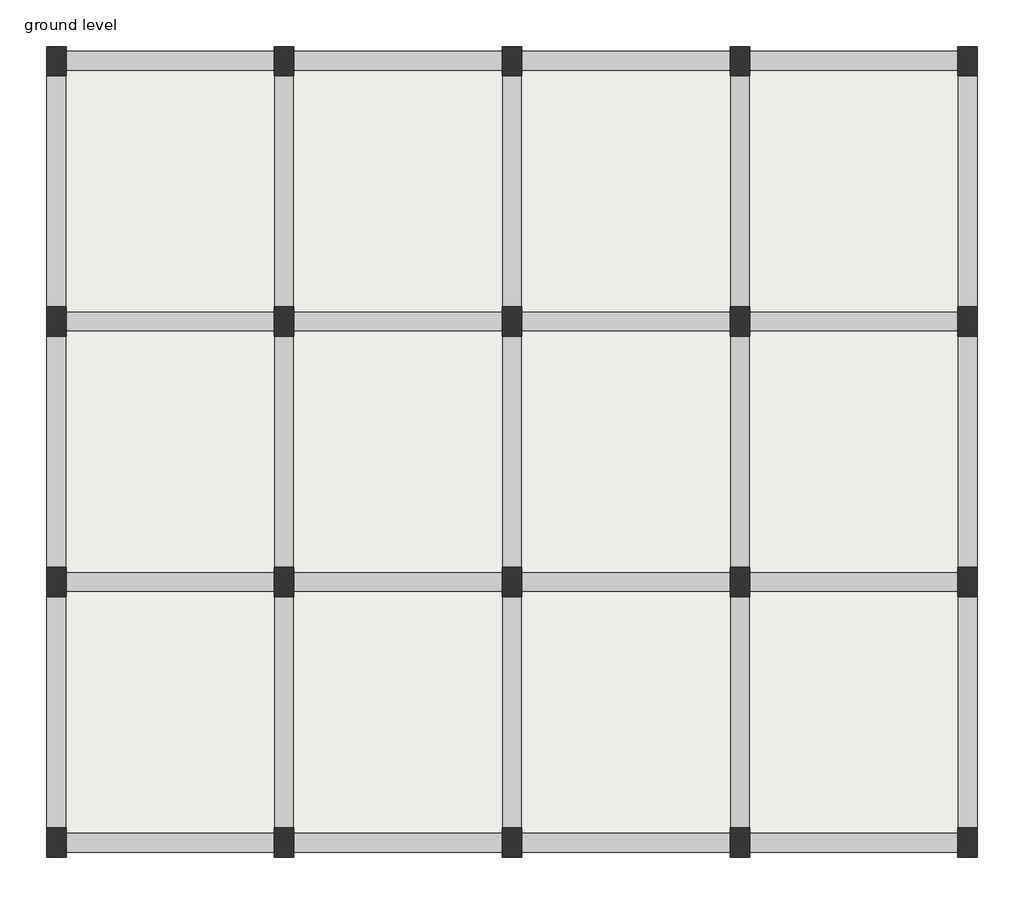
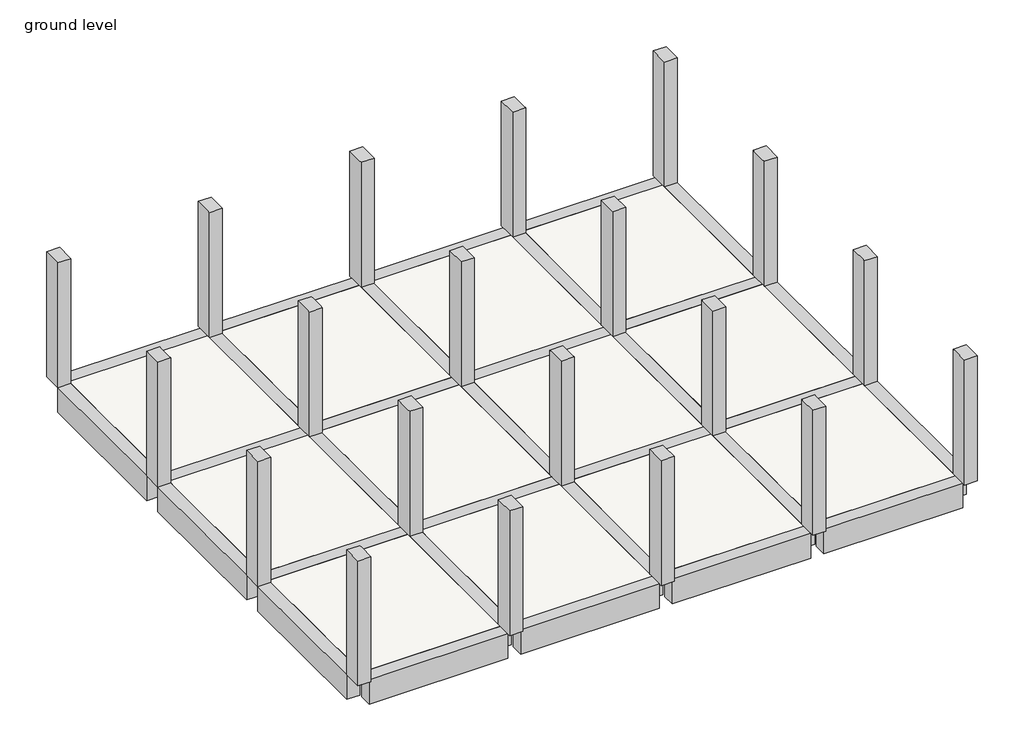
# One storey: 31 beams, 20 columns, 12 slabs.
"""IFC4 building model written with IfcOpenShell, lengths in millimetres."""

from ifc_helpers import new_model, si_unit, frame, origin, place, context, project, spatial, polyline, outline, extrude, faceted_brep, element, save

model = new_model("IFC4")

# Units and contexts
model_context = context("Model", 3, world=origin())
ifc_project = project(units=[si_unit("LENGTHUNIT", "METRE", prefix="MILLI")], contexts=[model_context])

# Site, building, storey
site = spatial("IfcSite", under=ifc_project)
building = spatial("IfcBuilding", under=site)
storey = spatial("IfcBuildingStorey", under=building, Name="ground level", Elevation=0.0)

# Beams
placement = place(None, origin())
element("IfcBeam", 1, ObjectType="M_Concrete-Rectangular Beam : 300 x 600mm", at=placement, inside=storey, context=model_context, shape_type="SweptSolid", body=[
    extrude(outline(polyline([(-11089.0800189, 5761.4575251), (-11389.0800189, 5761.4575251), (-11389.0800189, 9311.4575251), (-11089.0800189, 9311.4575251), (-11089.0800189, 5761.4575251)])), frame((0.0, 0.0, -600.0), z_axis=(0.0, 0.0, 1.0), x_axis=(1.0, 0.0, 0.0)), (0.0, 0.0, 1.0), 600.0),
])
element("IfcBeam", 2, ObjectType="M_Concrete-Rectangular Beam : 300 x 600mm", at=placement, inside=storey, context=model_context, shape_type="SweptSolid", body=[
    extrude(outline(polyline([(-11089.0800189, 9761.4575251), (-11389.0800189, 9761.4575251), (-11389.0800189, 13311.4575251), (-11089.0800189, 13311.4575251), (-11089.0800189, 9761.4575251)])), frame((0.0, 0.0, -600.0), z_axis=(0.0, 0.0, 1.0), x_axis=(1.0, 0.0, 0.0)), (0.0, 0.0, 1.0), 600.0),
])
element("IfcBeam", 3, ObjectType="M_Concrete-Rectangular Beam : 300 x 600mm", at=placement, inside=storey, context=model_context, shape_type="SweptSolid", body=[
    extrude(outline(polyline([(-11089.0800189, 13761.4575251), (-11389.0800189, 13761.4575251), (-11389.0800189, 17311.4575251), (-11089.0800189, 17311.4575251), (-11089.0800189, 13761.4575251)])), frame((0.0, 0.0, -600.0), z_axis=(0.0, 0.0, 1.0), x_axis=(1.0, 0.0, 0.0)), (0.0, 0.0, 1.0), 600.0),
])
element("IfcBeam", 4, ObjectType="M_Concrete-Rectangular Beam : 300 x 600mm", at=placement, inside=storey, context=model_context, shape_type="SweptSolid", body=[
    extrude(outline(polyline([(-7589.0800189, 5761.4575251), (-7889.0800189, 5761.4575251), (-7889.0800189, 9311.4575251), (-7589.0800189, 9311.4575251), (-7589.0800189, 5761.4575251)])), frame((0.0, 0.0, -600.0), z_axis=(0.0, 0.0, 1.0), x_axis=(1.0, 0.0, 0.0)), (0.0, 0.0, 1.0), 600.0),
])
element("IfcBeam", 5, ObjectType="M_Concrete-Rectangular Beam : 300 x 600mm", at=placement, inside=storey, context=model_context, shape_type="SweptSolid", body=[
    extrude(outline(polyline([(-7589.0800189, 9761.4575251), (-7889.0800189, 9761.4575251), (-7889.0800189, 13311.4575251), (-7589.0800189, 13311.4575251), (-7589.0800189, 9761.4575251)])), frame((0.0, 0.0, -600.0), z_axis=(0.0, 0.0, 1.0), x_axis=(1.0, 0.0, 0.0)), (0.0, 0.0, 1.0), 600.0),
])
element("IfcBeam", 6, ObjectType="M_Concrete-Rectangular Beam : 300 x 600mm", at=placement, inside=storey, context=model_context, shape_type="SweptSolid", body=[
    extrude(outline(polyline([(-7589.0800189, 13761.4575251), (-7889.0800189, 13761.4575251), (-7889.0800189, 17311.4575251), (-7589.0800189, 17311.4575251), (-7589.0800189, 13761.4575251)])), frame((0.0, 0.0, -600.0), z_axis=(0.0, 0.0, 1.0), x_axis=(1.0, 0.0, 0.0)), (0.0, 0.0, 1.0), 600.0),
])
element("IfcBeam", 7, ObjectType="M_Concrete-Rectangular Beam : 300 x 600mm", at=placement, inside=storey, context=model_context, shape_type="SweptSolid", body=[
    extrude(outline(polyline([(-4089.0800189, 5761.4575251), (-4389.0800189, 5761.4575251), (-4389.0800189, 9311.4575251), (-4089.0800189, 9311.4575251), (-4089.0800189, 5761.4575251)])), frame((0.0, 0.0, -600.0), z_axis=(0.0, 0.0, 1.0), x_axis=(1.0, 0.0, 0.0)), (0.0, 0.0, 1.0), 600.0),
])
element("IfcBeam", 8, ObjectType="M_Concrete-Rectangular Beam : 300 x 600mm", at=placement, inside=storey, context=model_context, shape_type="SweptSolid", body=[
    extrude(outline(polyline([(-4089.0800189, 9761.4575251), (-4389.0800189, 9761.4575251), (-4389.0800189, 13311.4575251), (-4089.0800189, 13311.4575251), (-4089.0800189, 9761.4575251)])), frame((0.0, 0.0, -600.0), z_axis=(0.0, 0.0, 1.0), x_axis=(1.0, 0.0, 0.0)), (0.0, 0.0, 1.0), 600.0),
])
element("IfcBeam", 9, ObjectType="M_Concrete-Rectangular Beam : 300 x 600mm", at=placement, inside=storey, context=model_context, shape_type="SweptSolid", body=[
    extrude(outline(polyline([(-4089.0800189, 13761.4575251), (-4389.0800189, 13761.4575251), (-4389.0800189, 17311.4575251), (-4089.0800189, 17311.4575251), (-4089.0800189, 13761.4575251)])), frame((0.0, 0.0, -600.0), z_axis=(0.0, 0.0, 1.0), x_axis=(1.0, 0.0, 0.0)), (0.0, 0.0, 1.0), 600.0),
])
element("IfcBeam", 10, ObjectType="M_Concrete-Rectangular Beam : 300 x 600mm", at=placement, inside=storey, context=model_context, shape_type="SweptSolid", body=[
    extrude(outline(polyline([(-589.0800189, 5761.4575251), (-889.0800189, 5761.4575251), (-889.0800189, 9311.4575251), (-589.0800189, 9311.4575251), (-589.0800189, 5761.4575251)])), frame((0.0, 0.0, -600.0), z_axis=(0.0, 0.0, 1.0), x_axis=(1.0, 0.0, 0.0)), (0.0, 0.0, 1.0), 600.0),
])
element("IfcBeam", 11, ObjectType="M_Concrete-Rectangular Beam : 300 x 600mm", at=placement, inside=storey, context=model_context, shape_type="SweptSolid", body=[
    extrude(outline(polyline([(-589.0800189, 9761.4575251), (-889.0800189, 9761.4575251), (-889.0800189, 13311.4575251), (-589.0800189, 13311.4575251), (-589.0800189, 9761.4575251)])), frame((0.0, 0.0, -600.0), z_axis=(0.0, 0.0, 1.0), x_axis=(1.0, 0.0, 0.0)), (0.0, 0.0, 1.0), 600.0),
])
element("IfcBeam", 12, ObjectType="M_Concrete-Rectangular Beam : 300 x 600mm", at=placement, inside=storey, context=model_context, shape_type="SweptSolid", body=[
    extrude(outline(polyline([(-589.0800189, 13761.4575251), (-889.0800189, 13761.4575251), (-889.0800189, 17311.4575251), (-589.0800189, 17311.4575251), (-589.0800189, 13761.4575251)])), frame((0.0, 0.0, -600.0), z_axis=(0.0, 0.0, 1.0), x_axis=(1.0, 0.0, 0.0)), (0.0, 0.0, 1.0), 600.0),
])
element("IfcBeam", 13, ObjectType="M_Concrete-Rectangular Beam : 300 x 600mm", at=placement, inside=storey, context=model_context, shape_type="SweptSolid", body=[
    extrude(outline(polyline([(2910.9199811, 5761.4575251), (2610.9199811, 5761.4575251), (2610.9199811, 9311.4575251), (2910.9199811, 9311.4575251), (2910.9199811, 5761.4575251)])), frame((0.0, 0.0, -600.0), z_axis=(0.0, 0.0, 1.0), x_axis=(1.0, 0.0, 0.0)), (0.0, 0.0, 1.0), 600.0),
])
element("IfcBeam", 14, ObjectType="M_Concrete-Rectangular Beam : 300 x 600mm", at=placement, inside=storey, context=model_context, shape_type="SweptSolid", body=[
    extrude(outline(polyline([(2910.9199811, 9761.4575251), (2610.9199811, 9761.4575251), (2610.9199811, 13311.4575251), (2910.9199811, 13311.4575251), (2910.9199811, 9761.4575251)])), frame((0.0, 0.0, -600.0), z_axis=(0.0, 0.0, 1.0), x_axis=(1.0, 0.0, 0.0)), (0.0, 0.0, 1.0), 600.0),
])
element("IfcBeam", 15, ObjectType="M_Concrete-Rectangular Beam : 300 x 600mm", at=placement, inside=storey, context=model_context, shape_type="SweptSolid", body=[
    extrude(outline(polyline([(2910.9199811, 13761.4575251), (2610.9199811, 13761.4575251), (2610.9199811, 17311.4575251), (2910.9199811, 17311.4575251), (2910.9199811, 13761.4575251)])), frame((0.0, 0.0, -600.0), z_axis=(0.0, 0.0, 1.0), x_axis=(1.0, 0.0, 0.0)), (0.0, 0.0, 1.0), 600.0),
])
element("IfcBeam", 16, ObjectType="M_Concrete-Rectangular Beam : 300 x 600mm", at=placement, inside=storey, context=model_context, shape_type="Brep", body=[
    faceted_brep([(-11089.0800189, 17686.4575251, 0.0), (-11089.0800189, 17386.4575251, 0.0), (-7889.0800189, 17386.4575251, 0.0), (-7889.0800189, 17686.4575251, 0.0), (-11089.0800189, 17386.4575251, -300.0), (-11089.0800189, 17386.4575251, -600.0), (-7889.0800189, 17386.4575251, -600.0), (-7889.0800189, 17386.4575251, -300.0), (-11089.0800189, 17686.4575251, -600.0), (-7889.0800189, 17686.4575251, -600.0)], [[[0, 1, 2, 3]], [[1, 4, 5, 6, 7, 2]], [[5, 8, 9, 6]], [[8, 0, 3, 9]], [[5, 4, 1, 0, 8]], [[2, 7, 6, 9, 3]]]),
])
element("IfcBeam", 17, ObjectType="M_Concrete-Rectangular Beam : 300 x 600mm", at=placement, inside=storey, context=model_context, shape_type="Brep", body=[
    faceted_brep([(-7589.0800189, 17686.4575251, 0.0), (-7589.0800189, 17386.4575251, 0.0), (-4389.0800189, 17386.4575251, 0.0), (-4389.0800189, 17686.4575251, 0.0), (-7589.0800189, 17386.4575251, -300.0), (-7589.0800189, 17386.4575251, -600.0), (-4389.0800189, 17386.4575251, -600.0), (-4389.0800189, 17386.4575251, -300.0), (-7589.0800189, 17686.4575251, -600.0), (-4389.0800189, 17686.4575251, -600.0)], [[[0, 1, 2, 3]], [[1, 4, 5, 6, 7, 2]], [[5, 8, 9, 6]], [[8, 0, 3, 9]], [[5, 4, 1, 0, 8]], [[2, 7, 6, 9, 3]]]),
])
element("IfcBeam", 18, ObjectType="M_Concrete-Rectangular Beam : 300 x 600mm", at=placement, inside=storey, context=model_context, shape_type="Brep", body=[
    faceted_brep([(-4089.0800189, 17686.4575251, 0.0), (-4089.0800189, 17386.4575251, 0.0), (-889.0800189, 17386.4575251, 0.0), (-889.0800189, 17686.4575251, 0.0), (-4089.0800189, 17386.4575251, -300.0), (-4089.0800189, 17386.4575251, -600.0), (-889.0800189, 17386.4575251, -600.0), (-889.0800189, 17386.4575251, -300.0), (-4089.0800189, 17686.4575251, -600.0), (-889.0800189, 17686.4575251, -600.0)], [[[0, 1, 2, 3]], [[1, 4, 5, 6, 7, 2]], [[5, 8, 9, 6]], [[8, 0, 3, 9]], [[5, 4, 1, 0, 8]], [[2, 7, 6, 9, 3]]]),
])
element("IfcBeam", 19, ObjectType="M_Concrete-Rectangular Beam : 300 x 600mm", at=placement, inside=storey, context=model_context, shape_type="Brep", body=[
    faceted_brep([(-589.0800189, 17686.4575251, 0.0), (-589.0800189, 17386.4575251, 0.0), (2610.9199811, 17386.4575251, 0.0), (2610.9199811, 17686.4575251, 0.0), (-589.0800189, 17386.4575251, -300.0), (-589.0800189, 17386.4575251, -600.0), (2610.9199811, 17386.4575251, -600.0), (2610.9199811, 17386.4575251, -300.0), (-589.0800189, 17686.4575251, -600.0), (2610.9199811, 17686.4575251, -600.0)], [[[0, 1, 2, 3]], [[1, 4, 5, 6, 7, 2]], [[5, 8, 9, 6]], [[8, 0, 3, 9]], [[5, 4, 1, 0, 8]], [[2, 7, 6, 9, 3]]]),
])
element("IfcBeam", 20, ObjectType="M_Concrete-Rectangular Beam : 300 x 600mm", at=placement, inside=storey, context=model_context, shape_type="Brep", body=[
    faceted_brep([(-11089.0800189, 13686.4575251, 0.0), (-11089.0800189, 13386.4575251, 0.0), (-7889.0800189, 13386.4575251, 0.0), (-7889.0800189, 13686.4575251, 0.0), (-11089.0800189, 13386.4575251, -300.0), (-11089.0800189, 13386.4575251, -600.0), (-7889.0800189, 13386.4575251, -600.0), (-7889.0800189, 13386.4575251, -300.0), (-11089.0800189, 13686.4575251, -600.0), (-7889.0800189, 13686.4575251, -600.0), (-11089.0800189, 13686.4575251, -300.0), (-7889.0800189, 13686.4575251, -300.0)], [[[0, 1, 2, 3]], [[1, 4, 5, 6, 7, 2]], [[5, 8, 9, 6]], [[8, 10, 0, 3, 11, 9]], [[5, 4, 1, 0, 10, 8]], [[2, 7, 6, 9, 11, 3]]]),
])
element("IfcBeam", 21, ObjectType="M_Concrete-Rectangular Beam : 300 x 600mm", at=placement, inside=storey, context=model_context, shape_type="Brep", body=[
    faceted_brep([(-7589.0800189, 13686.4575251, 0.0), (-7589.0800189, 13386.4575251, 0.0), (-4389.0800189, 13386.4575251, 0.0), (-4389.0800189, 13686.4575251, 0.0), (-7589.0800189, 13386.4575251, -300.0), (-7589.0800189, 13386.4575251, -600.0), (-4389.0800189, 13386.4575251, -600.0), (-4389.0800189, 13386.4575251, -300.0), (-7589.0800189, 13686.4575251, -600.0), (-4389.0800189, 13686.4575251, -600.0), (-7589.0800189, 13686.4575251, -300.0), (-4389.0800189, 13686.4575251, -300.0)], [[[0, 1, 2, 3]], [[1, 4, 5, 6, 7, 2]], [[5, 8, 9, 6]], [[8, 10, 0, 3, 11, 9]], [[5, 4, 1, 0, 10, 8]], [[2, 7, 6, 9, 11, 3]]]),
])
element("IfcBeam", 22, ObjectType="M_Concrete-Rectangular Beam : 300 x 600mm", at=placement, inside=storey, context=model_context, shape_type="Brep", body=[
    faceted_brep([(-4089.0800189, 13686.4575251, 0.0), (-4089.0800189, 13386.4575251, 0.0), (-889.0800189, 13386.4575251, 0.0), (-889.0800189, 13686.4575251, 0.0), (-4089.0800189, 13386.4575251, -300.0), (-4089.0800189, 13386.4575251, -600.0), (-889.0800189, 13386.4575251, -600.0), (-889.0800189, 13386.4575251, -300.0), (-4089.0800189, 13686.4575251, -600.0), (-889.0800189, 13686.4575251, -600.0), (-4089.0800189, 13686.4575251, -300.0), (-889.0800189, 13686.4575251, -300.0)], [[[0, 1, 2, 3]], [[1, 4, 5, 6, 7, 2]], [[5, 8, 9, 6]], [[8, 10, 0, 3, 11, 9]], [[5, 4, 1, 0, 10, 8]], [[2, 7, 6, 9, 11, 3]]]),
])
element("IfcBeam", 23, ObjectType="M_Concrete-Rectangular Beam : 300 x 600mm", at=placement, inside=storey, context=model_context, shape_type="Brep", body=[
    faceted_brep([(-589.0800189, 13686.4575251, 0.0), (-589.0800189, 13386.4575251, 0.0), (2610.9199811, 13386.4575251, 0.0), (2610.9199811, 13686.4575251, 0.0), (-589.0800189, 13386.4575251, -300.0), (-589.0800189, 13386.4575251, -600.0), (2610.9199811, 13386.4575251, -600.0), (2610.9199811, 13386.4575251, -300.0), (-589.0800189, 13686.4575251, -600.0), (2610.9199811, 13686.4575251, -600.0), (-589.0800189, 13686.4575251, -300.0), (2610.9199811, 13686.4575251, -300.0)], [[[0, 1, 2, 3]], [[1, 4, 5, 6, 7, 2]], [[5, 8, 9, 6]], [[8, 10, 0, 3, 11, 9]], [[5, 4, 1, 0, 10, 8]], [[2, 7, 6, 9, 11, 3]]]),
])
element("IfcBeam", 24, ObjectType="M_Concrete-Rectangular Beam : 300 x 600mm", at=placement, inside=storey, context=model_context, shape_type="Brep", body=[
    faceted_brep([(-11089.0800189, 9686.4575251, 0.0), (-11089.0800189, 9386.4575251, 0.0), (-7889.0800189, 9386.4575251, 0.0), (-7889.0800189, 9686.4575251, 0.0), (-11089.0800189, 9386.4575251, -300.0), (-11089.0800189, 9386.4575251, -600.0), (-7889.0800189, 9386.4575251, -600.0), (-7889.0800189, 9386.4575251, -300.0), (-11089.0800189, 9686.4575251, -600.0), (-7889.0800189, 9686.4575251, -600.0), (-11089.0800189, 9686.4575251, -300.0), (-7889.0800189, 9686.4575251, -300.0)], [[[0, 1, 2, 3]], [[1, 4, 5, 6, 7, 2]], [[5, 8, 9, 6]], [[8, 10, 0, 3, 11, 9]], [[5, 4, 1, 0, 10, 8]], [[2, 7, 6, 9, 11, 3]]]),
])
element("IfcBeam", 25, ObjectType="M_Concrete-Rectangular Beam : 300 x 600mm", at=placement, inside=storey, context=model_context, shape_type="Brep", body=[
    faceted_brep([(-7589.0800189, 9686.4575251, 0.0), (-7589.0800189, 9386.4575251, 0.0), (-4389.0800189, 9386.4575251, 0.0), (-4389.0800189, 9686.4575251, 0.0), (-7589.0800189, 9386.4575251, -300.0), (-7589.0800189, 9386.4575251, -600.0), (-4389.0800189, 9386.4575251, -600.0), (-4389.0800189, 9386.4575251, -300.0), (-7589.0800189, 9686.4575251, -600.0), (-4389.0800189, 9686.4575251, -600.0), (-7589.0800189, 9686.4575251, -300.0), (-4389.0800189, 9686.4575251, -300.0)], [[[0, 1, 2, 3]], [[1, 4, 5, 6, 7, 2]], [[5, 8, 9, 6]], [[8, 10, 0, 3, 11, 9]], [[5, 4, 1, 0, 10, 8]], [[2, 7, 6, 9, 11, 3]]]),
])
element("IfcBeam", 26, ObjectType="M_Concrete-Rectangular Beam : 300 x 600mm", at=placement, inside=storey, context=model_context, shape_type="Brep", body=[
    faceted_brep([(-4089.0800189, 9686.4575251, 0.0), (-4089.0800189, 9386.4575251, 0.0), (-889.0800189, 9386.4575251, 0.0), (-889.0800189, 9686.4575251, 0.0), (-4089.0800189, 9386.4575251, -300.0), (-4089.0800189, 9386.4575251, -600.0), (-889.0800189, 9386.4575251, -600.0), (-889.0800189, 9386.4575251, -300.0), (-4089.0800189, 9686.4575251, -600.0), (-889.0800189, 9686.4575251, -600.0), (-4089.0800189, 9686.4575251, -300.0), (-889.0800189, 9686.4575251, -300.0)], [[[0, 1, 2, 3]], [[1, 4, 5, 6, 7, 2]], [[5, 8, 9, 6]], [[8, 10, 0, 3, 11, 9]], [[5, 4, 1, 0, 10, 8]], [[2, 7, 6, 9, 11, 3]]]),
])
element("IfcBeam", 27, ObjectType="M_Concrete-Rectangular Beam : 300 x 600mm", at=placement, inside=storey, context=model_context, shape_type="Brep", body=[
    faceted_brep([(-589.0800189, 9686.4575251, 0.0), (-589.0800189, 9386.4575251, 0.0), (2610.9199811, 9386.4575251, 0.0), (2610.9199811, 9686.4575251, 0.0), (-589.0800189, 9386.4575251, -300.0), (-589.0800189, 9386.4575251, -600.0), (2610.9199811, 9386.4575251, -600.0), (2610.9199811, 9386.4575251, -300.0), (-589.0800189, 9686.4575251, -600.0), (2610.9199811, 9686.4575251, -600.0), (-589.0800189, 9686.4575251, -300.0), (2610.9199811, 9686.4575251, -300.0)], [[[0, 1, 2, 3]], [[1, 4, 5, 6, 7, 2]], [[5, 8, 9, 6]], [[8, 10, 0, 3, 11, 9]], [[5, 4, 1, 0, 10, 8]], [[2, 7, 6, 9, 11, 3]]]),
])
element("IfcBeam", 28, ObjectType="M_Concrete-Rectangular Beam : 300 x 600mm", at=placement, inside=storey, context=model_context, shape_type="Brep", body=[
    faceted_brep([(-11089.0800189, 5686.4575251, 0.0), (-11089.0800189, 5386.4575251, 0.0), (-7889.0800189, 5386.4575251, 0.0), (-7889.0800189, 5686.4575251, 0.0), (-11089.0800189, 5386.4575251, -600.0), (-7889.0800189, 5386.4575251, -600.0), (-11089.0800189, 5686.4575251, -600.0), (-7889.0800189, 5686.4575251, -600.0), (-11089.0800189, 5686.4575251, -300.0), (-7889.0800189, 5686.4575251, -300.0)], [[[0, 1, 2, 3]], [[1, 4, 5, 2]], [[4, 6, 7, 5]], [[6, 8, 0, 3, 9, 7]], [[0, 8, 6, 4, 1]], [[2, 5, 7, 9, 3]]]),
])
element("IfcBeam", 29, ObjectType="M_Concrete-Rectangular Beam : 300 x 600mm", at=placement, inside=storey, context=model_context, shape_type="Brep", body=[
    faceted_brep([(-7589.0800189, 5686.4575251, 0.0), (-7589.0800189, 5386.4575251, 0.0), (-4389.0800189, 5386.4575251, 0.0), (-4389.0800189, 5686.4575251, 0.0), (-7589.0800189, 5386.4575251, -600.0), (-4389.0800189, 5386.4575251, -600.0), (-7589.0800189, 5686.4575251, -600.0), (-4389.0800189, 5686.4575251, -600.0), (-7589.0800189, 5686.4575251, -300.0), (-4389.0800189, 5686.4575251, -300.0)], [[[0, 1, 2, 3]], [[1, 4, 5, 2]], [[4, 6, 7, 5]], [[6, 8, 0, 3, 9, 7]], [[0, 8, 6, 4, 1]], [[2, 5, 7, 9, 3]]]),
])
element("IfcBeam", 30, ObjectType="M_Concrete-Rectangular Beam : 300 x 600mm", at=placement, inside=storey, context=model_context, shape_type="Brep", body=[
    faceted_brep([(-4089.0800189, 5686.4575251, 0.0), (-4089.0800189, 5386.4575251, 0.0), (-889.0800189, 5386.4575251, 0.0), (-889.0800189, 5686.4575251, 0.0), (-4089.0800189, 5386.4575251, -600.0), (-889.0800189, 5386.4575251, -600.0), (-4089.0800189, 5686.4575251, -600.0), (-889.0800189, 5686.4575251, -600.0), (-4089.0800189, 5686.4575251, -300.0), (-889.0800189, 5686.4575251, -300.0)], [[[0, 1, 2, 3]], [[1, 4, 5, 2]], [[4, 6, 7, 5]], [[6, 8, 0, 3, 9, 7]], [[0, 8, 6, 4, 1]], [[2, 5, 7, 9, 3]]]),
])
element("IfcBeam", 31, ObjectType="M_Concrete-Rectangular Beam : 300 x 600mm", at=placement, inside=storey, context=model_context, shape_type="Brep", body=[
    faceted_brep([(-589.0800189, 5686.4575251, 0.0), (-589.0800189, 5386.4575251, 0.0), (2610.9199811, 5386.4575251, 0.0), (2610.9199811, 5686.4575251, 0.0), (-589.0800189, 5386.4575251, -600.0), (2610.9199811, 5386.4575251, -600.0), (-589.0800189, 5686.4575251, -600.0), (2610.9199811, 5686.4575251, -600.0), (-589.0800189, 5686.4575251, -300.0), (2610.9199811, 5686.4575251, -300.0)], [[[0, 1, 2, 3]], [[1, 4, 5, 2]], [[4, 6, 7, 5]], [[6, 8, 0, 3, 9, 7]], [[0, 8, 6, 4, 1]], [[2, 5, 7, 9, 3]]]),
])

# Columns
element("IfcColumn", 32, ObjectType="M_Concrete-Rectangular-Column : 300 x 450mm", at=placement, inside=storey, context=model_context, shape_type="Brep", body=[
    faceted_brep([(-11089.0800189, 17761.4575251, 0.0), (-11089.0800189, 17311.4575251, 0.0), (-11389.0800189, 17311.4575251, 0.0), (-11389.0800189, 17761.4575251, 0.0), (-11089.0800189, 17761.4575251, 3048.0), (-11089.0800189, 17386.4575251, 3048.0), (-11089.0800189, 17311.4575251, 3048.0), (-11389.0800189, 17311.4575251, 3048.0), (-11389.0800189, 17761.4575251, 3048.0)], [[[0, 1, 2, 3]], [[4, 5, 6, 1, 0]], [[6, 7, 2, 1]], [[7, 8, 3, 2]], [[8, 4, 0, 3]], [[4, 8, 7, 6, 5]]]),
])
element("IfcColumn", 33, ObjectType="M_Concrete-Rectangular-Column : 300 x 450mm", at=placement, inside=storey, context=model_context, shape_type="Brep", body=[
    faceted_brep([(-11089.0800189, 13761.4575251, 0.0), (-11089.0800189, 13311.4575251, 0.0), (-11389.0800189, 13311.4575251, 0.0), (-11389.0800189, 13761.4575251, 0.0), (-11089.0800189, 13761.4575251, 3048.0), (-11089.0800189, 13686.4575251, 3048.0), (-11089.0800189, 13386.4575251, 3048.0), (-11089.0800189, 13311.4575251, 3048.0), (-11389.0800189, 13311.4575251, 3048.0), (-11389.0800189, 13761.4575251, 3048.0)], [[[0, 1, 2, 3]], [[4, 5, 6, 7, 1, 0]], [[7, 8, 2, 1]], [[8, 9, 3, 2]], [[9, 4, 0, 3]], [[4, 9, 8, 7, 6, 5]]]),
])
element("IfcColumn", 34, ObjectType="M_Concrete-Rectangular-Column : 300 x 450mm", at=placement, inside=storey, context=model_context, shape_type="Brep", body=[
    faceted_brep([(-11089.0800189, 9761.4575251, 0.0), (-11089.0800189, 9311.4575251, 0.0), (-11389.0800189, 9311.4575251, 0.0), (-11389.0800189, 9761.4575251, 0.0), (-11089.0800189, 9761.4575251, 3048.0), (-11089.0800189, 9686.4575251, 3048.0), (-11089.0800189, 9386.4575251, 3048.0), (-11089.0800189, 9311.4575251, 3048.0), (-11389.0800189, 9311.4575251, 3048.0), (-11389.0800189, 9761.4575251, 3048.0)], [[[0, 1, 2, 3]], [[4, 5, 6, 7, 1, 0]], [[7, 8, 2, 1]], [[8, 9, 3, 2]], [[9, 4, 0, 3]], [[4, 9, 8, 7, 6, 5]]]),
])
element("IfcColumn", 35, ObjectType="M_Concrete-Rectangular-Column : 300 x 450mm", at=placement, inside=storey, context=model_context, shape_type="Brep", body=[
    faceted_brep([(-11089.0800189, 5761.4575251, 0.0), (-11089.0800189, 5311.4575251, 0.0), (-11389.0800189, 5311.4575251, 0.0), (-11389.0800189, 5761.4575251, 0.0), (-11089.0800189, 5761.4575251, 3048.0), (-11089.0800189, 5686.4575251, 3048.0), (-11089.0800189, 5311.4575251, 3048.0), (-11389.0800189, 5311.4575251, 3048.0), (-11389.0800189, 5761.4575251, 3048.0)], [[[0, 1, 2, 3]], [[4, 5, 6, 1, 0]], [[6, 7, 2, 1]], [[7, 8, 3, 2]], [[8, 4, 0, 3]], [[4, 8, 7, 6, 5]]]),
])
element("IfcColumn", 36, ObjectType="M_Concrete-Rectangular-Column : 300 x 450mm", at=placement, inside=storey, context=model_context, shape_type="Brep", body=[
    faceted_brep([(-7589.0800189, 17761.4575251, 0.0), (-7589.0800189, 17311.4575251, 0.0), (-7889.0800189, 17311.4575251, 0.0), (-7889.0800189, 17761.4575251, 0.0), (-7589.0800189, 17761.4575251, 3048.0), (-7589.0800189, 17386.4575251, 3048.0), (-7589.0800189, 17311.4575251, 3048.0), (-7889.0800189, 17311.4575251, 3048.0), (-7889.0800189, 17386.4575251, 3048.0), (-7889.0800189, 17761.4575251, 3048.0)], [[[0, 1, 2, 3]], [[4, 5, 6, 1, 0]], [[6, 7, 2, 1]], [[7, 8, 9, 3, 2]], [[9, 4, 0, 3]], [[4, 9, 8, 7, 6, 5]]]),
])
element("IfcColumn", 37, ObjectType="M_Concrete-Rectangular-Column : 300 x 450mm", at=placement, inside=storey, context=model_context, shape_type="Brep", body=[
    faceted_brep([(-7589.0800189, 13761.4575251, 0.0), (-7589.0800189, 13311.4575251, 0.0), (-7889.0800189, 13311.4575251, 0.0), (-7889.0800189, 13761.4575251, 0.0), (-7589.0800189, 13761.4575251, 3048.0), (-7589.0800189, 13686.4575251, 3048.0), (-7589.0800189, 13386.4575251, 3048.0), (-7589.0800189, 13311.4575251, 3048.0), (-7889.0800189, 13311.4575251, 3048.0), (-7889.0800189, 13386.4575251, 3048.0), (-7889.0800189, 13686.4575251, 3048.0), (-7889.0800189, 13761.4575251, 3048.0)], [[[0, 1, 2, 3]], [[4, 5, 6, 7, 1, 0]], [[7, 8, 2, 1]], [[8, 9, 10, 11, 3, 2]], [[11, 4, 0, 3]], [[4, 11, 10, 9, 8, 7, 6, 5]]]),
])
element("IfcColumn", 38, ObjectType="M_Concrete-Rectangular-Column : 300 x 450mm", at=placement, inside=storey, context=model_context, shape_type="Brep", body=[
    faceted_brep([(-7589.0800189, 9761.4575251, 0.0), (-7589.0800189, 9311.4575251, 0.0), (-7889.0800189, 9311.4575251, 0.0), (-7889.0800189, 9761.4575251, 0.0), (-7589.0800189, 9761.4575251, 3048.0), (-7589.0800189, 9686.4575251, 3048.0), (-7589.0800189, 9386.4575251, 3048.0), (-7589.0800189, 9311.4575251, 3048.0), (-7889.0800189, 9311.4575251, 3048.0), (-7889.0800189, 9386.4575251, 3048.0), (-7889.0800189, 9686.4575251, 3048.0), (-7889.0800189, 9761.4575251, 3048.0)], [[[0, 1, 2, 3]], [[4, 5, 6, 7, 1, 0]], [[7, 8, 2, 1]], [[8, 9, 10, 11, 3, 2]], [[11, 4, 0, 3]], [[4, 11, 10, 9, 8, 7, 6, 5]]]),
])
element("IfcColumn", 39, ObjectType="M_Concrete-Rectangular-Column : 300 x 450mm", at=placement, inside=storey, context=model_context, shape_type="Brep", body=[
    faceted_brep([(-7589.0800189, 5761.4575251, 0.0), (-7589.0800189, 5311.4575251, 0.0), (-7889.0800189, 5311.4575251, 0.0), (-7889.0800189, 5761.4575251, 0.0), (-7589.0800189, 5761.4575251, 3048.0), (-7589.0800189, 5686.4575251, 3048.0), (-7589.0800189, 5311.4575251, 3048.0), (-7889.0800189, 5311.4575251, 3048.0), (-7889.0800189, 5686.4575251, 3048.0), (-7889.0800189, 5761.4575251, 3048.0)], [[[0, 1, 2, 3]], [[4, 5, 6, 1, 0]], [[6, 7, 2, 1]], [[7, 8, 9, 3, 2]], [[9, 4, 0, 3]], [[4, 9, 8, 7, 6, 5]]]),
])
element("IfcColumn", 40, ObjectType="M_Concrete-Rectangular-Column : 300 x 450mm", at=placement, inside=storey, context=model_context, shape_type="Brep", body=[
    faceted_brep([(-4089.0800189, 17761.4575251, 0.0), (-4089.0800189, 17311.4575251, 0.0), (-4389.0800189, 17311.4575251, 0.0), (-4389.0800189, 17761.4575251, 0.0), (-4089.0800189, 17761.4575251, 3048.0), (-4089.0800189, 17386.4575251, 3048.0), (-4089.0800189, 17311.4575251, 3048.0), (-4389.0800189, 17311.4575251, 3048.0), (-4389.0800189, 17386.4575251, 3048.0), (-4389.0800189, 17761.4575251, 3048.0)], [[[0, 1, 2, 3]], [[4, 5, 6, 1, 0]], [[6, 7, 2, 1]], [[7, 8, 9, 3, 2]], [[9, 4, 0, 3]], [[4, 9, 8, 7, 6, 5]]]),
])
element("IfcColumn", 41, ObjectType="M_Concrete-Rectangular-Column : 300 x 450mm", at=placement, inside=storey, context=model_context, shape_type="Brep", body=[
    faceted_brep([(-4089.0800189, 13761.4575251, 0.0), (-4089.0800189, 13311.4575251, 0.0), (-4389.0800189, 13311.4575251, 0.0), (-4389.0800189, 13761.4575251, 0.0), (-4089.0800189, 13761.4575251, 3048.0), (-4089.0800189, 13686.4575251, 3048.0), (-4089.0800189, 13386.4575251, 3048.0), (-4089.0800189, 13311.4575251, 3048.0), (-4389.0800189, 13311.4575251, 3048.0), (-4389.0800189, 13386.4575251, 3048.0), (-4389.0800189, 13686.4575251, 3048.0), (-4389.0800189, 13761.4575251, 3048.0)], [[[0, 1, 2, 3]], [[4, 5, 6, 7, 1, 0]], [[7, 8, 2, 1]], [[8, 9, 10, 11, 3, 2]], [[11, 4, 0, 3]], [[4, 11, 10, 9, 8, 7, 6, 5]]]),
])
element("IfcColumn", 42, ObjectType="M_Concrete-Rectangular-Column : 300 x 450mm", at=placement, inside=storey, context=model_context, shape_type="Brep", body=[
    faceted_brep([(-4089.0800189, 9761.4575251, 0.0), (-4089.0800189, 9311.4575251, 0.0), (-4389.0800189, 9311.4575251, 0.0), (-4389.0800189, 9761.4575251, 0.0), (-4089.0800189, 9761.4575251, 3048.0), (-4089.0800189, 9686.4575251, 3048.0), (-4089.0800189, 9386.4575251, 3048.0), (-4089.0800189, 9311.4575251, 3048.0), (-4389.0800189, 9311.4575251, 3048.0), (-4389.0800189, 9386.4575251, 3048.0), (-4389.0800189, 9686.4575251, 3048.0), (-4389.0800189, 9761.4575251, 3048.0)], [[[0, 1, 2, 3]], [[4, 5, 6, 7, 1, 0]], [[7, 8, 2, 1]], [[8, 9, 10, 11, 3, 2]], [[11, 4, 0, 3]], [[4, 11, 10, 9, 8, 7, 6, 5]]]),
])
element("IfcColumn", 43, ObjectType="M_Concrete-Rectangular-Column : 300 x 450mm", at=placement, inside=storey, context=model_context, shape_type="Brep", body=[
    faceted_brep([(-4089.0800189, 5761.4575251, 0.0), (-4089.0800189, 5311.4575251, 0.0), (-4389.0800189, 5311.4575251, 0.0), (-4389.0800189, 5761.4575251, 0.0), (-4089.0800189, 5761.4575251, 3048.0), (-4089.0800189, 5686.4575251, 3048.0), (-4089.0800189, 5311.4575251, 3048.0), (-4389.0800189, 5311.4575251, 3048.0), (-4389.0800189, 5686.4575251, 3048.0), (-4389.0800189, 5761.4575251, 3048.0)], [[[0, 1, 2, 3]], [[4, 5, 6, 1, 0]], [[6, 7, 2, 1]], [[7, 8, 9, 3, 2]], [[9, 4, 0, 3]], [[4, 9, 8, 7, 6, 5]]]),
])
element("IfcColumn", 44, ObjectType="M_Concrete-Rectangular-Column : 300 x 450mm", at=placement, inside=storey, context=model_context, shape_type="Brep", body=[
    faceted_brep([(-589.0800189, 17761.4575251, 0.0), (-589.0800189, 17311.4575251, 0.0), (-889.0800189, 17311.4575251, 0.0), (-889.0800189, 17761.4575251, 0.0), (-589.0800189, 17761.4575251, 3048.0), (-589.0800189, 17386.4575251, 3048.0), (-589.0800189, 17311.4575251, 3048.0), (-889.0800189, 17311.4575251, 3048.0), (-889.0800189, 17386.4575251, 3048.0), (-889.0800189, 17761.4575251, 3048.0)], [[[0, 1, 2, 3]], [[4, 5, 6, 1, 0]], [[6, 7, 2, 1]], [[7, 8, 9, 3, 2]], [[9, 4, 0, 3]], [[4, 9, 8, 7, 6, 5]]]),
])
element("IfcColumn", 45, ObjectType="M_Concrete-Rectangular-Column : 300 x 450mm", at=placement, inside=storey, context=model_context, shape_type="Brep", body=[
    faceted_brep([(-589.0800189, 13761.4575251, 0.0), (-589.0800189, 13311.4575251, 0.0), (-889.0800189, 13311.4575251, 0.0), (-889.0800189, 13761.4575251, 0.0), (-589.0800189, 13761.4575251, 3048.0), (-589.0800189, 13686.4575251, 3048.0), (-589.0800189, 13386.4575251, 3048.0), (-589.0800189, 13311.4575251, 3048.0), (-889.0800189, 13311.4575251, 3048.0), (-889.0800189, 13386.4575251, 3048.0), (-889.0800189, 13686.4575251, 3048.0), (-889.0800189, 13761.4575251, 3048.0)], [[[0, 1, 2, 3]], [[4, 5, 6, 7, 1, 0]], [[7, 8, 2, 1]], [[8, 9, 10, 11, 3, 2]], [[11, 4, 0, 3]], [[4, 11, 10, 9, 8, 7, 6, 5]]]),
])
element("IfcColumn", 46, ObjectType="M_Concrete-Rectangular-Column : 300 x 450mm", at=placement, inside=storey, context=model_context, shape_type="Brep", body=[
    faceted_brep([(-589.0800189, 9761.4575251, 0.0), (-589.0800189, 9311.4575251, 0.0), (-889.0800189, 9311.4575251, 0.0), (-889.0800189, 9761.4575251, 0.0), (-589.0800189, 9761.4575251, 3048.0), (-589.0800189, 9686.4575251, 3048.0), (-589.0800189, 9386.4575251, 3048.0), (-589.0800189, 9311.4575251, 3048.0), (-889.0800189, 9311.4575251, 3048.0), (-889.0800189, 9386.4575251, 3048.0), (-889.0800189, 9686.4575251, 3048.0), (-889.0800189, 9761.4575251, 3048.0)], [[[0, 1, 2, 3]], [[4, 5, 6, 7, 1, 0]], [[7, 8, 2, 1]], [[8, 9, 10, 11, 3, 2]], [[11, 4, 0, 3]], [[4, 11, 10, 9, 8, 7, 6, 5]]]),
])
element("IfcColumn", 47, ObjectType="M_Concrete-Rectangular-Column : 300 x 450mm", at=placement, inside=storey, context=model_context, shape_type="Brep", body=[
    faceted_brep([(-589.0800189, 5761.4575251, 0.0), (-589.0800189, 5311.4575251, 0.0), (-889.0800189, 5311.4575251, 0.0), (-889.0800189, 5761.4575251, 0.0), (-589.0800189, 5761.4575251, 3048.0), (-589.0800189, 5686.4575251, 3048.0), (-589.0800189, 5311.4575251, 3048.0), (-889.0800189, 5311.4575251, 3048.0), (-889.0800189, 5686.4575251, 3048.0), (-889.0800189, 5761.4575251, 3048.0)], [[[0, 1, 2, 3]], [[4, 5, 6, 1, 0]], [[6, 7, 2, 1]], [[7, 8, 9, 3, 2]], [[9, 4, 0, 3]], [[4, 9, 8, 7, 6, 5]]]),
])
element("IfcColumn", 48, ObjectType="M_Concrete-Rectangular-Column : 300 x 450mm", at=placement, inside=storey, context=model_context, shape_type="Brep", body=[
    faceted_brep([(2910.9199811, 17761.4575251, 0.0), (2910.9199811, 17311.4575251, 0.0), (2610.9199811, 17311.4575251, 0.0), (2610.9199811, 17761.4575251, 0.0), (2910.9199811, 17761.4575251, 3048.0), (2910.9199811, 17311.4575251, 3048.0), (2610.9199811, 17311.4575251, 3048.0), (2610.9199811, 17386.4575251, 3048.0), (2610.9199811, 17761.4575251, 3048.0)], [[[0, 1, 2, 3]], [[4, 5, 1, 0]], [[5, 6, 2, 1]], [[6, 7, 8, 3, 2]], [[8, 4, 0, 3]], [[4, 8, 7, 6, 5]]]),
])
element("IfcColumn", 49, ObjectType="M_Concrete-Rectangular-Column : 300 x 450mm", at=placement, inside=storey, context=model_context, shape_type="Brep", body=[
    faceted_brep([(2910.9199811, 13761.4575251, 0.0), (2910.9199811, 13311.4575251, 0.0), (2610.9199811, 13311.4575251, 0.0), (2610.9199811, 13761.4575251, 0.0), (2910.9199811, 13761.4575251, 3048.0), (2910.9199811, 13311.4575251, 3048.0), (2610.9199811, 13311.4575251, 3048.0), (2610.9199811, 13386.4575251, 3048.0), (2610.9199811, 13686.4575251, 3048.0), (2610.9199811, 13761.4575251, 3048.0)], [[[0, 1, 2, 3]], [[4, 5, 1, 0]], [[5, 6, 2, 1]], [[6, 7, 8, 9, 3, 2]], [[9, 4, 0, 3]], [[4, 9, 8, 7, 6, 5]]]),
])
element("IfcColumn", 50, ObjectType="M_Concrete-Rectangular-Column : 300 x 450mm", at=placement, inside=storey, context=model_context, shape_type="Brep", body=[
    faceted_brep([(2910.9199811, 9761.4575251, 0.0), (2910.9199811, 9311.4575251, 0.0), (2610.9199811, 9311.4575251, 0.0), (2610.9199811, 9761.4575251, 0.0), (2910.9199811, 9761.4575251, 3048.0), (2910.9199811, 9311.4575251, 3048.0), (2610.9199811, 9311.4575251, 3048.0), (2610.9199811, 9386.4575251, 3048.0), (2610.9199811, 9686.4575251, 3048.0), (2610.9199811, 9761.4575251, 3048.0)], [[[0, 1, 2, 3]], [[4, 5, 1, 0]], [[5, 6, 2, 1]], [[6, 7, 8, 9, 3, 2]], [[9, 4, 0, 3]], [[4, 9, 8, 7, 6, 5]]]),
])
element("IfcColumn", 51, ObjectType="M_Concrete-Rectangular-Column : 300 x 450mm", at=placement, inside=storey, context=model_context, shape_type="Brep", body=[
    faceted_brep([(2910.9199811, 5761.4575251, 0.0), (2910.9199811, 5311.4575251, 0.0), (2610.9199811, 5311.4575251, 0.0), (2610.9199811, 5761.4575251, 0.0), (2910.9199811, 5761.4575251, 3048.0), (2910.9199811, 5311.4575251, 3048.0), (2610.9199811, 5311.4575251, 3048.0), (2610.9199811, 5686.4575251, 3048.0), (2610.9199811, 5761.4575251, 3048.0)], [[[0, 1, 2, 3]], [[4, 5, 1, 0]], [[5, 6, 2, 1]], [[6, 7, 8, 3, 2]], [[8, 4, 0, 3]], [[4, 8, 7, 6, 5]]]),
])

# Slabs
element("IfcSlab", 52, ObjectType="Generic 300mm", at=placement, inside=storey, context=model_context, shape_type="Brep", body=[
    faceted_brep([(-7889.0800189, 17386.4575251, -300.0), (-7889.0800189, 13686.4575251, -300.0), (-11089.0800189, 13686.4575251, -300.0), (-11089.0800189, 17386.4575251, -300.0), (-7889.0800189, 17386.4575251, 0.0), (-11089.0800189, 17386.4575251, 0.0), (-11089.0800189, 17311.4575251, 0.0), (-11089.0800189, 13761.4575251, 0.0), (-11089.0800189, 13686.4575251, 0.0), (-7889.0800189, 13686.4575251, 0.0), (-7889.0800189, 13761.4575251, 0.0), (-7889.0800189, 17311.4575251, 0.0)], [[[0, 1, 2, 3]], [[4, 5, 6, 7, 8, 9, 10, 11]], [[1, 0, 4, 11, 10, 9]], [[2, 1, 9, 8]], [[3, 2, 8, 7, 6, 5]], [[0, 3, 5, 4]]]),
])
element("IfcSlab", 53, ObjectType="Generic 300mm", at=placement, inside=storey, context=model_context, shape_type="Brep", body=[
    faceted_brep([(-4389.0800189, 17386.4575251, -300.0), (-4389.0800189, 13686.4575251, -300.0), (-7589.0800189, 13686.4575251, -300.0), (-7589.0800189, 17386.4575251, -300.0), (-4389.0800189, 17386.4575251, 0.0), (-7589.0800189, 17386.4575251, 0.0), (-7589.0800189, 17311.4575251, 0.0), (-7589.0800189, 13761.4575251, 0.0), (-7589.0800189, 13686.4575251, 0.0), (-4389.0800189, 13686.4575251, 0.0), (-4389.0800189, 13761.4575251, 0.0), (-4389.0800189, 17311.4575251, 0.0)], [[[0, 1, 2, 3]], [[4, 5, 6, 7, 8, 9, 10, 11]], [[1, 0, 4, 11, 10, 9]], [[2, 1, 9, 8]], [[3, 2, 8, 7, 6, 5]], [[0, 3, 5, 4]]]),
])
element("IfcSlab", 54, ObjectType="Generic 300mm", at=placement, inside=storey, context=model_context, shape_type="Brep", body=[
    faceted_brep([(-889.0800189, 17386.4575251, -300.0), (-889.0800189, 13686.4575251, -300.0), (-4089.0800189, 13686.4575251, -300.0), (-4089.0800189, 17386.4575251, -300.0), (-889.0800189, 17386.4575251, 0.0), (-4089.0800189, 17386.4575251, 0.0), (-4089.0800189, 17311.4575251, 0.0), (-4089.0800189, 13761.4575251, 0.0), (-4089.0800189, 13686.4575251, 0.0), (-889.0800189, 13686.4575251, 0.0), (-889.0800189, 13761.4575251, 0.0), (-889.0800189, 17311.4575251, 0.0)], [[[0, 1, 2, 3]], [[4, 5, 6, 7, 8, 9, 10, 11]], [[1, 0, 4, 11, 10, 9]], [[2, 1, 9, 8]], [[3, 2, 8, 7, 6, 5]], [[0, 3, 5, 4]]]),
])
element("IfcSlab", 55, ObjectType="Generic 300mm", at=placement, inside=storey, context=model_context, shape_type="Brep", body=[
    faceted_brep([(2610.9199811, 17386.4575251, -300.0), (2610.9199811, 13686.4575251, -300.0), (-589.0800189, 13686.4575251, -300.0), (-589.0800189, 17386.4575251, -300.0), (2610.9199811, 17386.4575251, 0.0), (-589.0800189, 17386.4575251, 0.0), (-589.0800189, 17311.4575251, 0.0), (-589.0800189, 13761.4575251, 0.0), (-589.0800189, 13686.4575251, 0.0), (2610.9199811, 13686.4575251, 0.0), (2610.9199811, 13761.4575251, 0.0), (2610.9199811, 17311.4575251, 0.0)], [[[0, 1, 2, 3]], [[4, 5, 6, 7, 8, 9, 10, 11]], [[1, 0, 4, 11, 10, 9]], [[2, 1, 9, 8]], [[3, 2, 8, 7, 6, 5]], [[0, 3, 5, 4]]]),
])
element("IfcSlab", 56, ObjectType="Generic 300mm", at=placement, inside=storey, context=model_context, shape_type="Brep", body=[
    faceted_brep([(2610.9199811, 13386.4575251, -300.0), (2610.9199811, 9686.4575251, -300.0), (-589.0800189, 9686.4575251, -300.0), (-589.0800189, 13386.4575251, -300.0), (2610.9199811, 13386.4575251, 0.0), (-589.0800189, 13386.4575251, 0.0), (-589.0800189, 13311.4575251, 0.0), (-589.0800189, 9761.4575251, 0.0), (-589.0800189, 9686.4575251, 0.0), (2610.9199811, 9686.4575251, 0.0), (2610.9199811, 9761.4575251, 0.0), (2610.9199811, 13311.4575251, 0.0)], [[[0, 1, 2, 3]], [[4, 5, 6, 7, 8, 9, 10, 11]], [[1, 0, 4, 11, 10, 9]], [[2, 1, 9, 8]], [[3, 2, 8, 7, 6, 5]], [[0, 3, 5, 4]]]),
])
element("IfcSlab", 57, ObjectType="Generic 300mm", at=placement, inside=storey, context=model_context, shape_type="Brep", body=[
    faceted_brep([(2610.9199811, 9386.4575251, -300.0), (2610.9199811, 5686.4575251, -300.0), (-589.0800189, 5686.4575251, -300.0), (-589.0800189, 9386.4575251, -300.0), (2610.9199811, 9386.4575251, 0.0), (-589.0800189, 9386.4575251, 0.0), (-589.0800189, 9311.4575251, 0.0), (-589.0800189, 5761.4575251, 0.0), (-589.0800189, 5686.4575251, 0.0), (2610.9199811, 5686.4575251, 0.0), (2610.9199811, 5761.4575251, 0.0), (2610.9199811, 9311.4575251, 0.0)], [[[0, 1, 2, 3]], [[4, 5, 6, 7, 8, 9, 10, 11]], [[1, 0, 4, 11, 10, 9]], [[2, 1, 9, 8]], [[3, 2, 8, 7, 6, 5]], [[0, 3, 5, 4]]]),
])
element("IfcSlab", 58, ObjectType="Generic 300mm", at=placement, inside=storey, context=model_context, shape_type="Brep", body=[
    faceted_brep([(-889.0800189, 9386.4575251, -300.0), (-889.0800189, 5686.4575251, -300.0), (-4089.0800189, 5686.4575251, -300.0), (-4089.0800189, 9386.4575251, -300.0), (-889.0800189, 9386.4575251, 0.0), (-4089.0800189, 9386.4575251, 0.0), (-4089.0800189, 9311.4575251, 0.0), (-4089.0800189, 5761.4575251, 0.0), (-4089.0800189, 5686.4575251, 0.0), (-889.0800189, 5686.4575251, 0.0), (-889.0800189, 5761.4575251, 0.0), (-889.0800189, 9311.4575251, 0.0)], [[[0, 1, 2, 3]], [[4, 5, 6, 7, 8, 9, 10, 11]], [[1, 0, 4, 11, 10, 9]], [[2, 1, 9, 8]], [[3, 2, 8, 7, 6, 5]], [[0, 3, 5, 4]]]),
])
element("IfcSlab", 59, ObjectType="Generic 300mm", at=placement, inside=storey, context=model_context, shape_type="Brep", body=[
    faceted_brep([(-4389.0800189, 9386.4575251, -300.0), (-4389.0800189, 5686.4575251, -300.0), (-7589.0800189, 5686.4575251, -300.0), (-7589.0800189, 9386.4575251, -300.0), (-4389.0800189, 9386.4575251, 0.0), (-7589.0800189, 9386.4575251, 0.0), (-7589.0800189, 9311.4575251, 0.0), (-7589.0800189, 5761.4575251, 0.0), (-7589.0800189, 5686.4575251, 0.0), (-4389.0800189, 5686.4575251, 0.0), (-4389.0800189, 5761.4575251, 0.0), (-4389.0800189, 9311.4575251, 0.0)], [[[0, 1, 2, 3]], [[4, 5, 6, 7, 8, 9, 10, 11]], [[1, 0, 4, 11, 10, 9]], [[2, 1, 9, 8]], [[3, 2, 8, 7, 6, 5]], [[0, 3, 5, 4]]]),
])
element("IfcSlab", 60, ObjectType="Generic 300mm", at=placement, inside=storey, context=model_context, shape_type="Brep", body=[
    faceted_brep([(-7889.0800189, 9386.4575251, -300.0), (-7889.0800189, 5686.4575251, -300.0), (-11089.0800189, 5686.4575251, -300.0), (-11089.0800189, 9386.4575251, -300.0), (-7889.0800189, 9386.4575251, 0.0), (-11089.0800189, 9386.4575251, 0.0), (-11089.0800189, 9311.4575251, 0.0), (-11089.0800189, 5761.4575251, 0.0), (-11089.0800189, 5686.4575251, 0.0), (-7889.0800189, 5686.4575251, 0.0), (-7889.0800189, 5761.4575251, 0.0), (-7889.0800189, 9311.4575251, 0.0)], [[[0, 1, 2, 3]], [[4, 5, 6, 7, 8, 9, 10, 11]], [[1, 0, 4, 11, 10, 9]], [[2, 1, 9, 8]], [[3, 2, 8, 7, 6, 5]], [[0, 3, 5, 4]]]),
])
element("IfcSlab", 61, ObjectType="Generic 300mm", at=placement, inside=storey, context=model_context, shape_type="Brep", body=[
    faceted_brep([(-7889.0800189, 13386.4575251, -300.0), (-7889.0800189, 9686.4575251, -300.0), (-11089.0800189, 9686.4575251, -300.0), (-11089.0800189, 13386.4575251, -300.0), (-7889.0800189, 13386.4575251, 0.0), (-11089.0800189, 13386.4575251, 0.0), (-11089.0800189, 13311.4575251, 0.0), (-11089.0800189, 9761.4575251, 0.0), (-11089.0800189, 9686.4575251, 0.0), (-7889.0800189, 9686.4575251, 0.0), (-7889.0800189, 9761.4575251, 0.0), (-7889.0800189, 13311.4575251, 0.0)], [[[0, 1, 2, 3]], [[4, 5, 6, 7, 8, 9, 10, 11]], [[1, 0, 4, 11, 10, 9]], [[2, 1, 9, 8]], [[3, 2, 8, 7, 6, 5]], [[0, 3, 5, 4]]]),
])
element("IfcSlab", 62, ObjectType="Generic 300mm", at=placement, inside=storey, context=model_context, shape_type="Brep", body=[
    faceted_brep([(-4389.0800189, 13386.4575251, -300.0), (-4389.0800189, 9686.4575251, -300.0), (-7589.0800189, 9686.4575251, -300.0), (-7589.0800189, 13386.4575251, -300.0), (-4389.0800189, 13386.4575251, 0.0), (-7589.0800189, 13386.4575251, 0.0), (-7589.0800189, 13311.4575251, 0.0), (-7589.0800189, 9761.4575251, 0.0), (-7589.0800189, 9686.4575251, 0.0), (-4389.0800189, 9686.4575251, 0.0), (-4389.0800189, 9761.4575251, 0.0), (-4389.0800189, 13311.4575251, 0.0)], [[[0, 1, 2, 3]], [[4, 5, 6, 7, 8, 9, 10, 11]], [[1, 0, 4, 11, 10, 9]], [[2, 1, 9, 8]], [[3, 2, 8, 7, 6, 5]], [[0, 3, 5, 4]]]),
])
element("IfcSlab", 63, ObjectType="Generic 300mm", at=placement, inside=storey, context=model_context, shape_type="Brep", body=[
    faceted_brep([(-889.0800189, 13386.4575251, -300.0), (-889.0800189, 9686.4575251, -300.0), (-4089.0800189, 9686.4575251, -300.0), (-4089.0800189, 13386.4575251, -300.0), (-889.0800189, 13386.4575251, 0.0), (-4089.0800189, 13386.4575251, 0.0), (-4089.0800189, 13311.4575251, 0.0), (-4089.0800189, 9761.4575251, 0.0), (-4089.0800189, 9686.4575251, 0.0), (-889.0800189, 9686.4575251, 0.0), (-889.0800189, 9761.4575251, 0.0), (-889.0800189, 13311.4575251, 0.0)], [[[0, 1, 2, 3]], [[4, 5, 6, 7, 8, 9, 10, 11]], [[1, 0, 4, 11, 10, 9]], [[2, 1, 9, 8]], [[3, 2, 8, 7, 6, 5]], [[0, 3, 5, 4]]]),
])

save(model, "model.ifc")

# Revit data of these elements
# Type "M_Concrete-Rectangular Beam : 300 x 600mm"
#   Length [instance default] = 5' - 0"
#   b = 0' - 11.81102"
#   h = 1' - 11.62205"
#   Structural Material [instance default] = Concrete, Cast-in-Place gray
#   Assembly Code = ""
# Type "M_Concrete-Rectangular-Column : 300 x 450mm"
#   b = 0' - 11.81102"
#   h = 1' - 5.71654"
#   Structural Material [instance default] = Concrete, Cast-in-Place gray
# Type "Generic 300mm"
#   Function = 0
#   Layers, outside or top first: 0' - 11.81102" no material (function 1)
# Elements 1, 2, 3, 4, 5, 6, 7, 8, 9, 10, 11, 12, 13, 14, 15, 16, 17, 18, 19, 20, 21, 22, 23, 24, 25, 26, 27, 28, 29, 30, 31 (IfcBeam, "M_Concrete-Rectangular Beam : 300 x 600mm")
#   Phase Created = New Construction
#   Materials on its faces: "Concrete, Cast-in-Place gray"
# Elements 32, 33, 34, 35, 36, 37, 38, 39, 40, 41, 42, 43, 44, 45, 46, 47, 48, 49, 50, 51 (IfcColumn, "M_Concrete-Rectangular-Column : 300 x 450mm")
#   Structural Material = Concrete, Cast-in-Place gray
#   Phase Created = New Construction
#   Materials on its faces: "Concrete, Cast-in-Place gray"
# Elements 52, 53, 54, 55, 56, 57, 58, 59, 60, 61, 62, 63 (IfcSlab, "Generic 300mm")
#   Height Offset From Level = 0' - 0"
#   built-in parameter 1001954 = 1
#   Phase Created = New Construction
#   Materials on its faces: "Default Floor"
# Materials
#   "Concrete, Cast-in-Place gray": class "Concrete", colour RGB 192 192 192, transparency 0, Description = "Cast-in-place concrete", Cost = 0
#   "Default Floor": colour RGB 127 127 127, transparency 0, Cost = 0
